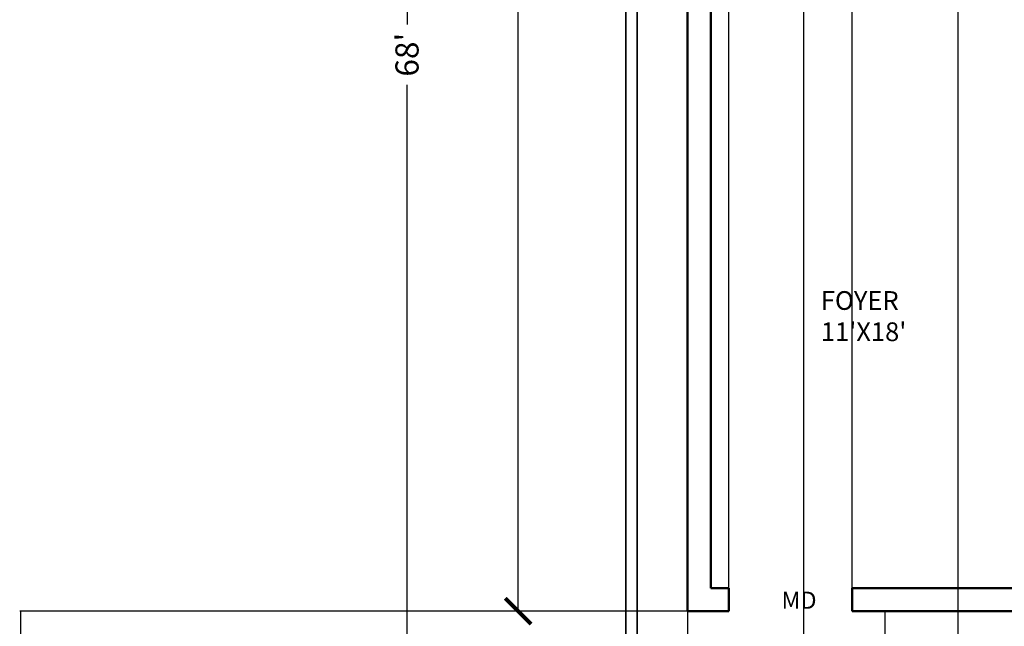
# Model space of a CAD drawing. Units: inches. Extents: x 338 to 1188, y -996 to 127.
# Tile 2 of 15: x 338 to 720, y -622 to -386. Entities that reach past the tile are written whole.
import ezdxf

# ---------------------------------------------------------------- set-up
doc = ezdxf.new("R2010")
doc.units = ezdxf.units.IN
doc.header["$MEASUREMENT"] = 0
for name, color, linetype, lineweight in [('A-ANNO-DIMS', 5, 'Continuous', 18), ('A-ANNO-TEXT', 7, 'Continuous', 18), ('A-AREA-IDEN', 8, 'Continuous', 18), ('A-FLOR-STRS', 7, 'Continuous', 25), ('C-PROP', 1, 'Continuous', 35), ('wall', 1, 'Continuous', 50)]:
    doc.layers.add(name, color=color, linetype=linetype, lineweight=lineweight)
doc.styles.get("Standard").update_dxf_attribs({"font": 'arial.ttf'})
doc.dimstyles.get("Standard").update_dxf_attribs({"dimtxt": 0.18, "dimasz": 0.18, "dimexe": 0.18, "dimexo": 0.0625, "dimgap": 0.09, "dimtad": 0, "dimtih": 1, "dimtoh": 1, "dimdec": 1, "dimzin": 0, "dimdsep": 46, "dimlunit": 4, "dimtxsty": 'Standard', "dimcen": 0.09, "dimadec": 0, "dimazin": 0, "dimtfac": 1, "dimtdec": 1, "dimtofl": 0, "dimtmove": 0, "dimatfit": 3, "dimfxl": 1, "dimtolj": 1, "dimtzin": 0, "dimarcsym": 0})

# ---------------------------------------------------------------- blocks, each defined once
blk = doc.blocks.new('_ArchTick')
at = {"color": 0, "linetype": 'ByBlock', "const_width": 0.15}
blk.add_lwpolyline([(-0.5, -0.5), (0.5, 0.5)], dxfattribs=at)
blk = doc.blocks.new('*D6')
at = {"layer": 'A-ANNO-DIMS', "color": 0, "lineweight": -2, "transparency": 16777216}
for p, q in [((531.19, -15.73), (531.19, -304.1)), ((531.19, -615.73), (531.19, -327.37))]:
    blk.add_line(p, q, dxfattribs=at)
at = {"layer": 'Defpoints', "color": 0, "transparency": 16777216}
for p in [(596.96, -15.73), (531.19, -615.73), (596.96, -615.73)]:
    blk.add_point(p, dxfattribs=at)
at = {"layer": 'A-ANNO-DIMS', "color": 0, "lineweight": -2, "transparency": 16777216, "xscale": 10, "yscale": 10, "zscale": 10}
for p, rotation in [((531.19, -15.73), 90), ((531.19, -615.73), 270)]:
    blk.add_blockref('_ArchTick', p, dxfattribs=dict(at, rotation=rotation))
at = {"layer": 'A-ANNO-DIMS', "color": 0, "transparency": 16777216, "insert": (531.19, -315.73), "char_height": 9, "attachment_point": 5, "rotation": 90}
blk.add_mtext("\\A1;50'", dxfattribs=at)
blk = doc.blocks.new('*D7')
at = {"layer": 'A-ANNO-DIMS', "color": 0, "lineweight": -2, "transparency": 16777216}
for p, q in [((488.01, 8.27), (488.01, -388.07)), ((488.01, -807.73), (488.01, -411.39))]:
    blk.add_line(p, q, dxfattribs=at)
at = {"layer": 'Defpoints', "color": 0, "transparency": 16777216}
for p in [(572.96, 8.27), (488.01, -807.73), (572.96, -807.73)]:
    blk.add_point(p, dxfattribs=at)
at = {"layer": 'A-ANNO-DIMS', "color": 0, "lineweight": -2, "transparency": 16777216, "xscale": 10, "yscale": 10, "zscale": 10}
for p, rotation in [((488.01, 8.27), 90), ((488.01, -807.73), 270)]:
    blk.add_blockref('_ArchTick', p, dxfattribs=dict(at, rotation=rotation))
at = {"layer": 'A-ANNO-DIMS', "color": 0, "transparency": 16777216, "insert": (488.01, -399.73), "char_height": 9, "attachment_point": 5, "rotation": 90}
blk.add_mtext("\\A1;68'", dxfattribs=at)
blk = doc.blocks.new('*D22')
at = {"layer": 'A-ANNO-DIMS', "color": 0, "lineweight": -2, "transparency": 16777216}
for p, q in [((596.9, -615.73), (337.66, -615.73)), ((337.84, -615.91), (337.84, -633.55)), ((337.84, -651.55), (337.84, -633.92)), ((596.9, -651.73), (337.66, -651.73))]:
    blk.add_line(p, q, dxfattribs=at)
at = {"layer": 'A-ANNO-DIMS', "color": 0, "transparency": 16777216}
for points in [[(337.81, -615.91), (337.87, -615.91), (337.84, -615.73)], [(337.81, -651.55), (337.87, -651.55), (337.84, -651.73)]]:
    blk.add_solid(points, dxfattribs=at)
at = {"layer": 'Defpoints', "color": 0, "transparency": 16777216}
for p in [(596.96, -615.73), (337.84, -651.73), (596.96, -651.73)]:
    blk.add_point(p, dxfattribs=at)
at = {"layer": 'A-ANNO-DIMS', "color": 0, "transparency": 16777216, "insert": (337.84, -633.73), "char_height": 0.18, "attachment_point": 5}
blk.add_mtext('\\A1;3\'-0"', dxfattribs=at)
blk = doc.blocks.new('*D31')
at = {"layer": 'A-ANNO-DIMS', "color": 0, "lineweight": -2, "transparency": 16777216}
for p, q in [((641.96, -149.3), (641.96, -968.86)), ((701.96, -149.3), (701.96, -968.86)), ((642.14, -968.68), (671.63, -968.68)), ((701.78, -968.68), (672.29, -968.68))]:
    blk.add_line(p, q, dxfattribs=at)
at = {"layer": 'A-ANNO-DIMS', "color": 0, "transparency": 16777216}
for points in [[(642.14, -968.65), (642.14, -968.71), (641.96, -968.68)], [(701.78, -968.65), (701.78, -968.71), (701.96, -968.68)]]:
    blk.add_solid(points, dxfattribs=at)
at = {"layer": 'Defpoints', "color": 0, "transparency": 16777216}
for p in [(641.96, -149.23), (701.96, -149.23), (701.96, -968.68)]:
    blk.add_point(p, dxfattribs=at)
at = {"layer": 'A-ANNO-DIMS', "color": 0, "transparency": 16777216, "insert": (671.96, -968.68), "char_height": 0.18, "attachment_point": 5}
blk.add_mtext('\\A1;5\'-0"', dxfattribs=at)
blk = doc.blocks.new('*D34')
at = {"layer": 'A-ANNO-DIMS', "color": 0, "lineweight": -2, "transparency": 16777216}
for p, q in [((612.96, -615.67), (612.96, 67.25)), ((613.14, 67.07), (636.63, 67.07)), ((660.78, 67.07), (637.3, 67.07)), ((660.96, -615.67), (660.96, 67.25))]:
    blk.add_line(p, q, dxfattribs=at)
at = {"layer": 'A-ANNO-DIMS', "color": 0, "transparency": 16777216}
for points in [[(613.14, 67.1), (613.14, 67.04), (612.96, 67.07)], [(660.78, 67.1), (660.78, 67.04), (660.96, 67.07)]]:
    blk.add_solid(points, dxfattribs=at)
at = {"layer": 'Defpoints', "color": 0, "transparency": 16777216}
for p in [(660.96, 67.07), (612.96, -615.73), (660.96, -615.73)]:
    blk.add_point(p, dxfattribs=at)
at = {"layer": 'A-ANNO-DIMS', "color": 0, "transparency": 16777216, "insert": (636.96, 67.07), "char_height": 0.18, "attachment_point": 5}
blk.add_mtext('\\A1;4\'-0"', dxfattribs=at)
blk = doc.blocks.new('*D48')
at = {"layer": 'A-ANNO-DIMS', "color": 0, "lineweight": -2, "transparency": 16777216}
for p, q in [((596.96, -615.67), (596.96, 67.25)), ((597.14, 67.07), (604.64, 67.07)), ((612.78, 67.07), (605.28, 67.07)), ((612.96, -615.67), (612.96, 67.25))]:
    blk.add_line(p, q, dxfattribs=at)
at = {"layer": 'A-ANNO-DIMS', "color": 0, "transparency": 16777216}
for points in [[(597.14, 67.1), (597.14, 67.04), (596.96, 67.07)], [(612.78, 67.1), (612.78, 67.04), (612.96, 67.07)]]:
    blk.add_solid(points, dxfattribs=at)
at = {"layer": 'Defpoints', "color": 0, "transparency": 16777216}
for p in [(612.96, 67.07), (596.96, -615.73), (612.96, -615.73)]:
    blk.add_point(p, dxfattribs=at)
at = {"layer": 'A-ANNO-DIMS', "color": 0, "transparency": 16777216, "insert": (604.96, 67.07), "char_height": 0.18, "attachment_point": 5}
blk.add_mtext('\\A1;1\'-4"', dxfattribs=at)

msp = doc.modelspace()

# ---------------------------------------------------------------- linework, layer by layer
at = {"layer": 'A-FLOR-STRS'}
for p, q in [((596.96, -615.73), (596.96, -651.73)), ((673.79, -651.73), (673.79, -615.73))]:
    msp.add_line(p, q, dxfattribs=at)
at = {"layer": 'C-PROP'}
for p, q in [((572.96, 8.27), (572.96, -807.73)), ((577.46, 3.77), (577.46, -803.23))]:
    msp.add_line(p, q, dxfattribs=at)
at = {"layer": 'wall'}
for p, q in [((596.96, -15.73), (596.96, -615.73)), ((605.96, -149.23), (605.96, -606.73)), ((612.96, -606.73), (605.96, -606.73)), ((612.96, -606.73), (612.96, -615.73)), ((737.96, -606.73), (660.96, -606.73)), ((660.96, -606.73), (660.96, -615.73)), ((612.96, -615.73), (596.96, -615.73)), ((956.96, -615.73), (660.96, -615.73))]:
    msp.add_line(p, q, dxfattribs=at)

# ---------------------------------------------------------------- texts
at = {"layer": 'A-ANNO-TEXT'}
msp.add_text('MD', height=6.652, dxfattribs=at).set_placement((633.48, -614.8))
at = {"layer": 'A-AREA-IDEN', "insert": (639.86, -491.51), "char_height": 7.2703, "attachment_point": 1}
msp.add_mtext_dynamic_manual_height_columns("    FOYER\\P    11'X18'", width=52.2141, gutter_width=1, heights=[0], dxfattribs=at)

# ---------------------------------------------------------------- dimensions: what is measured, and where the dimension line sits
at = {"layer": 'A-ANNO-DIMS'}
for base, p1, p2, picture, middle in [((612.96, 67.07), (596.96, -615.73), (612.96, -615.73), '*D48', (604.96, 67.07)), ((660.96, 67.07), (612.96, -615.73), (660.96, -615.73), '*D34', (636.96, 67.07)), ((701.96, -968.68), (641.96, -149.23), (701.96, -149.23), '*D31', (671.96, -968.68))]:
    dim = msp.add_linear_dim(base=base, p1=p1, p2=p2, dimstyle='Standard', override={"dimdec": 1, "dimlfac": 1, "dimrnd": 0, "dimzin": 1, "dimdsep": 46, "dimlunit": 4, "dimfrac": 2}, dxfattribs=at)
    dim.commit()
    dim.dimension.update_dxf_attribs({"geometry": picture, "text_midpoint": middle})
for base, p1, p2, override, picture, middle in [((488.01, -807.73), (572.96, 8.27), (572.96, -807.73), {"dimtxt": 9, "dimasz": 10, "dimgap": 4, "dimtad": 0, "dimtih": 0, "dimblk1": 'ArchTick', "dimblk2": 'ArchTick', "dimsah": 1, "dimse1": 1, "dimse2": 1, "dimclrd": 0, "dimclre": 0, "dimclrt": 0}, '*D7', (488.01, -399.73)), ((531.19, -615.73), (596.96, -15.73), (596.96, -615.73), {"dimtxt": 9, "dimasz": 10, "dimgap": 4, "dimtih": 0, "dimblk1": 'ArchTick', "dimblk2": 'ArchTick', "dimsah": 1, "dimse1": 1, "dimse2": 1, "dimclrd": 0, "dimclre": 0, "dimclrt": 0}, '*D6', (531.19, -315.73)), ((337.84, -651.73), (596.96, -615.73), (596.96, -651.73), {"dimdec": 1, "dimlfac": 1, "dimrnd": 0, "dimzin": 1, "dimdsep": 46, "dimlunit": 4, "dimfrac": 2}, '*D22', (337.84, -633.73))]:
    dim = msp.add_linear_dim(base=base, p1=p1, p2=p2, angle=90, dimstyle='Standard', override=override, dxfattribs=at)
    dim.commit()
    dim.dimension.update_dxf_attribs({"geometry": picture, "text_midpoint": middle})

doc.saveas('drawing.dxf')
